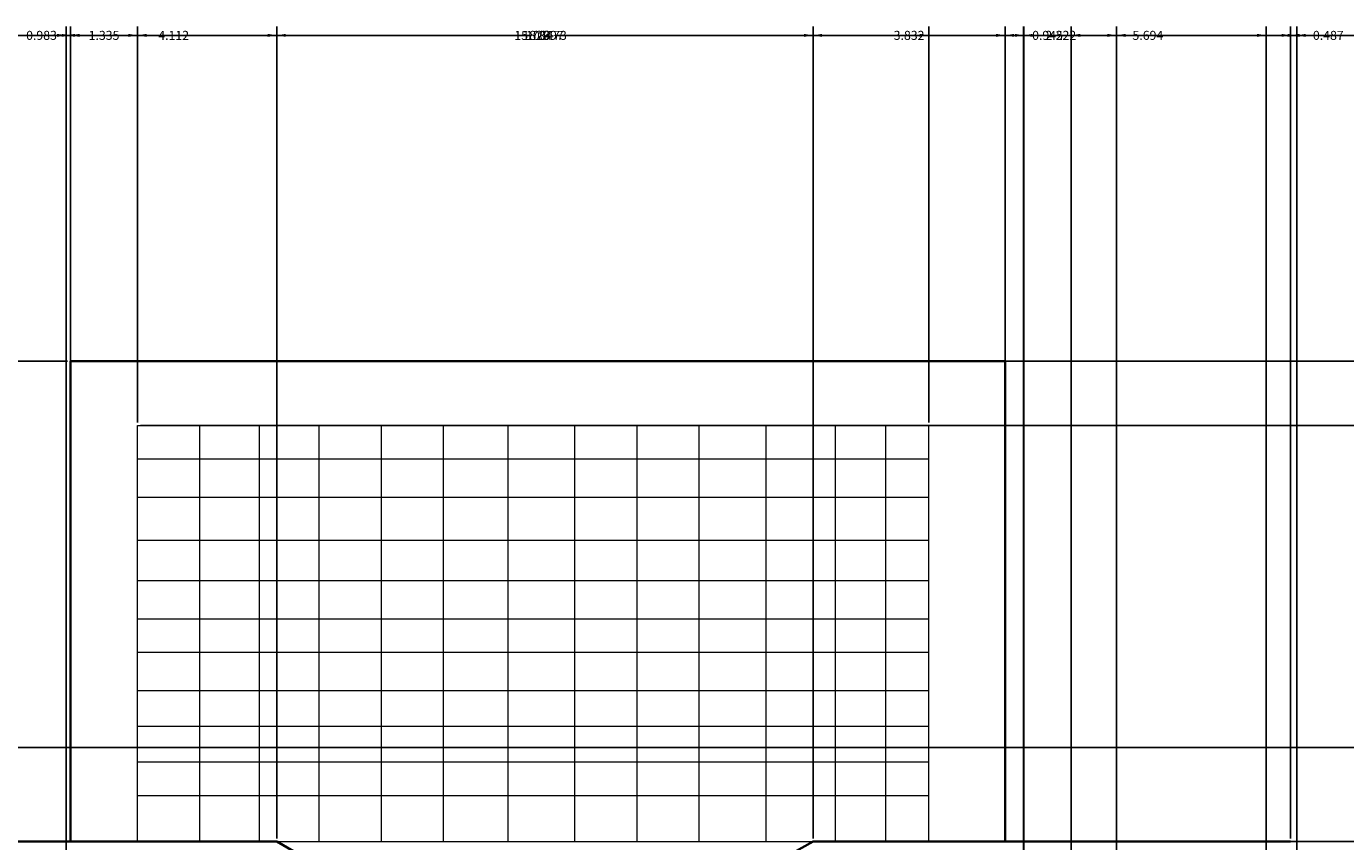
# Model space of a CAD drawing. Units: inches. Extents: x -10 to 130, y -32 to 34.
# Tile 17 of 22: x 49 to 75, y 18 to 34. Entities that reach past the tile are written whole.
import ezdxf

# ---------------------------------------------------------------- set-up
doc = ezdxf.new("R2010")
doc.units = ezdxf.units.IN
doc.header["$MEASUREMENT"] = 0
for name, color, linetype, lineweight in [('A-ANNO-DIMS', 2, 'Continuous', 18), ('A-ELEV', 7, 'Continuous', 35), ('A-GLAZ', 4, 'Continuous', 18)]:
    doc.layers.add(name, color=color, linetype=linetype, lineweight=lineweight)
doc.styles.get("Standard").update_dxf_attribs({"font": 'arial.ttf'})
doc.dimstyles.get("Standard").update_dxf_attribs({"dimtxt": 0.18, "dimasz": 0.18, "dimexe": 0.18, "dimexo": 0.0625, "dimgap": 0.09, "dimtad": 0, "dimtih": 1, "dimtoh": 1, "dimdec": 4, "dimzin": 0, "dimdsep": 46, "dimtxsty": 'Standard', "dimcen": 0.09, "dimadec": 0, "dimazin": 0, "dimtfac": 1, "dimtdec": 4, "dimtofl": 0, "dimtmove": 0, "dimatfit": 3, "dimfxl": 1, "dimtolj": 1, "dimtzin": 0, "dimarcsym": 0})

# ---------------------------------------------------------------- blocks, each defined once
blk = doc.blocks.new('*D2')
at = {"layer": 'A-ANNO-DIMS', "color": 0, "lineweight": -2, "transparency": 16777216}
for p, q in [((68.738, 27.199), (129.508, 27.199)), ((129.328, 27.019), (129.328, 3.074)), ((129.328, -21.234), (129.328, 2.71)), ((107.996, -21.414), (129.508, -21.414))]:
    blk.add_line(p, q, dxfattribs=at)
at = {"layer": 'A-ANNO-DIMS', "color": 0, "transparency": 16777216}
for points in [[(129.298, 27.019), (129.358, 27.019), (129.328, 27.199)], [(129.298, -21.234), (129.358, -21.234), (129.328, -21.414)]]:
    blk.add_solid(points, dxfattribs=at)
at = {"layer": 'Defpoints', "color": 0, "transparency": 16777216}
for p in [(68.676, 27.199), (129.328, 27.199), (107.933, -21.414)]:
    blk.add_point(p, dxfattribs=at)
at = {"layer": 'A-ANNO-DIMS', "color": 0, "transparency": 16777216, "insert": (129.328, 2.892), "char_height": 0.18, "attachment_point": 5}
blk.add_mtext('\\A1;48.61', dxfattribs=at)
blk = doc.blocks.new('*D7')
at = {"layer": 'A-ANNO-DIMS', "color": 0, "lineweight": -2, "transparency": 16777216}
for p, q in [((42.614, 6.07), (42.614, 33.879)), ((42.794, 33.699), (45.888, 33.699)), ((49.766, 33.699), (46.672, 33.699)), ((49.946, 6.07), (49.946, 33.879))]:
    blk.add_line(p, q, dxfattribs=at)
at = {"layer": 'A-ANNO-DIMS', "color": 0, "transparency": 16777216}
for points in [[(42.794, 33.729), (42.794, 33.669), (42.614, 33.699)], [(49.766, 33.729), (49.766, 33.669), (49.946, 33.699)]]:
    blk.add_solid(points, dxfattribs=at)
at = {"layer": 'Defpoints', "color": 0, "transparency": 16777216}
for p in [(49.946, 33.699), (42.614, 6.007), (49.946, 6.007)]:
    blk.add_point(p, dxfattribs=at)
at = {"layer": 'A-ANNO-DIMS', "color": 0, "transparency": 16777216, "insert": (46.28, 33.699), "char_height": 0.18, "attachment_point": 5}
blk.add_mtext('\\A1;7.332', dxfattribs=at)
blk = doc.blocks.new('*D8')
at = {"layer": 'A-ANNO-DIMS', "color": 0, "lineweight": -2, "transparency": 16777216}
for p, q in [((68.676, 17.67), (68.676, 33.879)), ((68.856, 33.699), (69.393, 33.699)), ((70.718, 33.699), (70.181, 33.699)), ((70.898, 6.07), (70.898, 33.879))]:
    blk.add_line(p, q, dxfattribs=at)
at = {"layer": 'A-ANNO-DIMS', "color": 0, "transparency": 16777216}
for points in [[(68.856, 33.729), (68.856, 33.669), (68.676, 33.699)], [(70.718, 33.729), (70.718, 33.669), (70.898, 33.699)]]:
    blk.add_solid(points, dxfattribs=at)
at = {"layer": 'Defpoints', "color": 0, "transparency": 16777216}
for p in [(70.898, 33.699), (68.676, 17.607), (70.898, 6.007)]:
    blk.add_point(p, dxfattribs=at)
at = {"layer": 'A-ANNO-DIMS', "color": 0, "transparency": 16777216, "insert": (69.787, 33.699), "char_height": 0.18, "attachment_point": 5}
blk.add_mtext('\\A1;2.222', dxfattribs=at)
blk = doc.blocks.new('*D9')
at = {"layer": 'A-ANNO-DIMS', "color": 0, "lineweight": -2, "transparency": 16777216}
for p, q in [((70.898, 6.07), (70.898, 33.879)), ((71.078, 33.699), (75.697, 33.699)), ((81.225, 33.699), (76.607, 33.699)), ((81.405, 6.07), (81.405, 33.879))]:
    blk.add_line(p, q, dxfattribs=at)
at = {"layer": 'A-ANNO-DIMS', "color": 0, "transparency": 16777216}
for points in [[(71.078, 33.729), (71.078, 33.669), (70.898, 33.699)], [(81.225, 33.729), (81.225, 33.669), (81.405, 33.699)]]:
    blk.add_solid(points, dxfattribs=at)
at = {"layer": 'Defpoints', "color": 0, "transparency": 16777216}
for p in [(81.405, 33.699), (70.898, 6.007), (81.405, 6.007)]:
    blk.add_point(p, dxfattribs=at)
at = {"layer": 'A-ANNO-DIMS', "color": 0, "transparency": 16777216, "insert": (76.152, 33.699), "char_height": 0.18, "attachment_point": 5}
blk.add_mtext('\\A1;10.507', dxfattribs=at)
blk = doc.blocks.new('*D18')
at = {"layer": 'A-ANNO-DIMS', "color": 0, "lineweight": -2, "transparency": 16777216}
for p, q in [((44.622, 17.67), (44.622, 33.879)), ((44.802, 33.699), (46.935, 33.699)), ((49.855, 33.699), (47.722, 33.699)), ((50.035, 27.261), (50.035, 33.879))]:
    blk.add_line(p, q, dxfattribs=at)
at = {"layer": 'A-ANNO-DIMS', "color": 0, "transparency": 16777216}
for points in [[(44.802, 33.729), (44.802, 33.669), (44.622, 33.699)], [(49.855, 33.729), (49.855, 33.669), (50.035, 33.699)]]:
    blk.add_solid(points, dxfattribs=at)
at = {"layer": 'Defpoints', "color": 0, "transparency": 16777216}
for p in [(50.035, 33.699), (50.035, 27.199), (44.622, 17.607)]:
    blk.add_point(p, dxfattribs=at)
at = {"layer": 'A-ANNO-DIMS', "color": 0, "transparency": 16777216, "insert": (47.328, 33.699), "char_height": 0.18, "attachment_point": 5}
blk.add_mtext('\\A1;5.413', dxfattribs=at)
blk = doc.blocks.new('*D19')
at = {"layer": 'A-ANNO-DIMS', "color": 0, "lineweight": -2, "transparency": 16777216}
for p, q in [((50.035, 27.261), (50.035, 33.879)), ((50.215, 33.699), (58.97, 33.699)), ((68.496, 33.699), (59.74, 33.699)), ((68.676, 27.261), (68.676, 33.879))]:
    blk.add_line(p, q, dxfattribs=at)
at = {"layer": 'A-ANNO-DIMS', "color": 0, "transparency": 16777216}
for points in [[(50.215, 33.729), (50.215, 33.669), (50.035, 33.699)], [(68.496, 33.729), (68.496, 33.669), (68.676, 33.699)]]:
    blk.add_solid(points, dxfattribs=at)
at = {"layer": 'Defpoints', "color": 0, "transparency": 16777216}
for p in [(68.676, 33.699), (50.035, 27.199), (68.676, 27.199)]:
    blk.add_point(p, dxfattribs=at)
at = {"layer": 'A-ANNO-DIMS', "color": 0, "transparency": 16777216, "insert": (59.355, 33.699), "char_height": 0.18, "attachment_point": 5}
blk.add_mtext('\\A1;18.64', dxfattribs=at)
blk = doc.blocks.new('*D20')
at = {"layer": 'A-ANNO-DIMS', "color": 0, "lineweight": -2, "transparency": 16777216}
for p, q in [((68.676, 27.261), (68.676, 33.879)), ((68.856, 33.699), (71.129, 33.699)), ((74.19, 33.699), (71.916, 33.699)), ((74.37, 17.67), (74.37, 33.879))]:
    blk.add_line(p, q, dxfattribs=at)
at = {"layer": 'A-ANNO-DIMS', "color": 0, "transparency": 16777216}
for points in [[(68.856, 33.729), (68.856, 33.669), (68.676, 33.699)], [(74.19, 33.729), (74.19, 33.669), (74.37, 33.699)]]:
    blk.add_solid(points, dxfattribs=at)
at = {"layer": 'Defpoints', "color": 0, "transparency": 16777216}
for p in [(74.37, 33.699), (68.676, 27.199), (74.37, 17.607)]:
    blk.add_point(p, dxfattribs=at)
at = {"layer": 'A-ANNO-DIMS', "color": 0, "transparency": 16777216, "insert": (71.523, 33.699), "char_height": 0.18, "attachment_point": 5}
blk.add_mtext('\\A1;5.694', dxfattribs=at)
blk = doc.blocks.new('*D21')
at = {"layer": 'A-ANNO-DIMS', "color": 0, "lineweight": -2, "transparency": 16777216}
for p, q in [((74.37, 17.67), (74.37, 33.879)), ((74.55, 33.699), (76.605, 33.699)), ((79.447, 33.699), (77.392, 33.699)), ((79.627, 19.52), (79.627, 33.879))]:
    blk.add_line(p, q, dxfattribs=at)
at = {"layer": 'A-ANNO-DIMS', "color": 0, "transparency": 16777216}
for points in [[(74.55, 33.729), (74.55, 33.669), (74.37, 33.699)], [(79.447, 33.729), (79.447, 33.669), (79.627, 33.699)]]:
    blk.add_solid(points, dxfattribs=at)
at = {"layer": 'Defpoints', "color": 0, "transparency": 16777216}
for p in [(79.627, 33.699), (79.627, 19.458), (74.37, 17.607)]:
    blk.add_point(p, dxfattribs=at)
at = {"layer": 'A-ANNO-DIMS', "color": 0, "transparency": 16777216, "insert": (76.998, 33.699), "char_height": 0.18, "attachment_point": 5}
blk.add_mtext('\\A1;5.257', dxfattribs=at)
blk = doc.blocks.new('*D28')
at = {"layer": 'A-ANNO-DIMS', "color": 0, "lineweight": -2, "transparency": 16777216}
for p, q in [((21.715, 14.903), (21.715, 33.879)), ((21.895, 33.699), (35.436, 33.699)), ((49.766, 33.699), (36.226, 33.699)), ((49.946, 14.903), (49.946, 33.879))]:
    blk.add_line(p, q, dxfattribs=at)
at = {"layer": 'A-ANNO-DIMS', "color": 0, "transparency": 16777216}
for points in [[(21.895, 33.729), (21.895, 33.669), (21.715, 33.699)], [(49.766, 33.729), (49.766, 33.669), (49.946, 33.699)]]:
    blk.add_solid(points, dxfattribs=at)
at = {"layer": 'Defpoints', "color": 0, "transparency": 16777216}
for p in [(49.946, 33.699), (21.715, 14.841), (49.946, 14.841)]:
    blk.add_point(p, dxfattribs=at)
at = {"layer": 'A-ANNO-DIMS', "color": 0, "transparency": 16777216, "insert": (35.831, 33.699), "char_height": 0.18, "attachment_point": 5}
blk.add_mtext('\\A1;28.23', dxfattribs=at)
blk = doc.blocks.new('*D29')
at = {"layer": 'A-ANNO-DIMS', "color": 0, "lineweight": -2, "transparency": 16777216}
for p, q in [((69.045, 14.903), (69.045, 33.879)), ((69.225, 33.699), (82.743, 33.699)), ((97.053, 33.699), (83.534, 33.699)), ((97.233, 14.903), (97.233, 33.879))]:
    blk.add_line(p, q, dxfattribs=at)
at = {"layer": 'A-ANNO-DIMS', "color": 0, "transparency": 16777216}
for points in [[(69.225, 33.729), (69.225, 33.669), (69.045, 33.699)], [(97.053, 33.729), (97.053, 33.669), (97.233, 33.699)]]:
    blk.add_solid(points, dxfattribs=at)
at = {"layer": 'Defpoints', "color": 0, "transparency": 16777216}
for p in [(97.233, 33.699), (69.045, 14.841), (97.233, 14.841)]:
    blk.add_point(p, dxfattribs=at)
at = {"layer": 'A-ANNO-DIMS', "color": 0, "transparency": 16777216, "insert": (83.139, 33.699), "char_height": 0.18, "attachment_point": 5}
blk.add_mtext('\\A1;28.19', dxfattribs=at)
blk = doc.blocks.new('*D39')
at = {"layer": 'A-ANNO-DIMS', "color": 0, "lineweight": -2, "transparency": 16777216}
for p, q in [((49.972, 27.199), (-9.564, 27.199)), ((-9.384, 27.019), (-9.384, 25.982)), ((-9.384, 24.582), (-9.384, 25.618)), ((28.037, 24.402), (-9.564, 24.402))]:
    blk.add_line(p, q, dxfattribs=at)
at = {"layer": 'A-ANNO-DIMS', "color": 0, "transparency": 16777216}
for points in [[(-9.414, 27.019), (-9.354, 27.019), (-9.384, 27.199)], [(-9.414, 24.582), (-9.354, 24.582), (-9.384, 24.402)]]:
    blk.add_solid(points, dxfattribs=at)
at = {"layer": 'Defpoints', "color": 0, "transparency": 16777216}
for p in [(-9.384, 27.199), (50.035, 27.199), (28.1, 24.402)]:
    blk.add_point(p, dxfattribs=at)
at = {"layer": 'A-ANNO-DIMS', "color": 0, "transparency": 16777216, "insert": (-9.384, 25.8), "char_height": 0.18, "attachment_point": 5}
blk.add_mtext('\\A1;2.797', dxfattribs=at)
blk = doc.blocks.new('*D48')
at = {"layer": 'A-ANNO-DIMS', "color": 0, "lineweight": -2, "transparency": 16777216}
for p, q in [((44.76, -13.293), (44.76, 33.879)), ((44.94, 33.699), (59.231, 33.699)), ((74.312, 33.699), (60.021, 33.699)), ((74.492, -13.293), (74.492, 33.879))]:
    blk.add_line(p, q, dxfattribs=at)
at = {"layer": 'A-ANNO-DIMS', "color": 0, "transparency": 16777216}
for points in [[(44.94, 33.729), (44.94, 33.669), (44.76, 33.699)], [(74.312, 33.729), (74.312, 33.669), (74.492, 33.699)]]:
    blk.add_solid(points, dxfattribs=at)
at = {"layer": 'Defpoints', "color": 0, "transparency": 16777216}
for p in [(74.492, 33.699), (44.76, -13.356), (74.492, -13.356)]:
    blk.add_point(p, dxfattribs=at)
at = {"layer": 'A-ANNO-DIMS', "color": 0, "transparency": 16777216, "insert": (59.626, 33.699), "char_height": 0.18, "attachment_point": 5}
blk.add_mtext('\\A1;29.73', dxfattribs=at)
blk = doc.blocks.new('*D60')
at = {"layer": 'A-ANNO-DIMS', "color": 0, "lineweight": -2, "transparency": 16777216}
for p, q in [((74.492, -13.293), (74.492, 33.879)), ((74.672, 33.699), (78.041, 33.699)), ((82.197, 33.699), (78.828, 33.699)), ((82.377, -15.202), (82.377, 33.879))]:
    blk.add_line(p, q, dxfattribs=at)
at = {"layer": 'A-ANNO-DIMS', "color": 0, "transparency": 16777216}
for points in [[(74.672, 33.729), (74.672, 33.669), (74.492, 33.699)], [(82.197, 33.729), (82.197, 33.669), (82.377, 33.699)]]:
    blk.add_solid(points, dxfattribs=at)
at = {"layer": 'Defpoints', "color": 0, "transparency": 16777216}
for p in [(82.377, 33.699), (74.492, -13.356), (82.377, -15.264)]:
    blk.add_point(p, dxfattribs=at)
at = {"layer": 'A-ANNO-DIMS', "color": 0, "transparency": 16777216, "insert": (78.435, 33.699), "char_height": 0.18, "attachment_point": 5}
blk.add_mtext('\\A1;7.885', dxfattribs=at)
blk = doc.blocks.new('*D70')
at = {"layer": 'A-ANNO-DIMS', "color": 0, "lineweight": -2, "transparency": 16777216}
for p, q in [((50.035, 17.67), (50.035, 33.879)), ((50.215, 33.699), (51.695, 33.699)), ((53.967, 33.699), (52.487, 33.699)), ((54.147, 17.67), (54.147, 33.879))]:
    blk.add_line(p, q, dxfattribs=at)
at = {"layer": 'A-ANNO-DIMS', "color": 0, "transparency": 16777216}
for points in [[(50.215, 33.729), (50.215, 33.669), (50.035, 33.699)], [(53.967, 33.729), (53.967, 33.669), (54.147, 33.699)]]:
    blk.add_solid(points, dxfattribs=at)
at = {"layer": 'Defpoints', "color": 0, "transparency": 16777216}
for p in [(54.147, 33.699), (50.035, 17.607), (54.147, 17.607)]:
    blk.add_point(p, dxfattribs=at)
at = {"layer": 'A-ANNO-DIMS', "color": 0, "transparency": 16777216, "insert": (52.091, 33.699), "char_height": 0.18, "attachment_point": 5}
blk.add_mtext('\\A1;4.112', dxfattribs=at)
blk = doc.blocks.new('*D71')
at = {"layer": 'A-ANNO-DIMS', "color": 0, "lineweight": -2, "transparency": 16777216}
for p, q in [((54.147, 17.67), (54.147, 33.879)), ((54.327, 33.699), (59.041, 33.699)), ((64.664, 33.699), (59.951, 33.699)), ((64.844, 17.67), (64.844, 33.879))]:
    blk.add_line(p, q, dxfattribs=at)
at = {"layer": 'A-ANNO-DIMS', "color": 0, "transparency": 16777216}
for points in [[(54.327, 33.729), (54.327, 33.669), (54.147, 33.699)], [(64.664, 33.729), (64.664, 33.669), (64.844, 33.699)]]:
    blk.add_solid(points, dxfattribs=at)
at = {"layer": 'Defpoints', "color": 0, "transparency": 16777216}
for p in [(64.844, 33.699), (54.147, 17.607), (64.844, 17.607)]:
    blk.add_point(p, dxfattribs=at)
at = {"layer": 'A-ANNO-DIMS', "color": 0, "transparency": 16777216, "insert": (59.496, 33.699), "char_height": 0.18, "attachment_point": 5}
blk.add_mtext('\\A1;10.697', dxfattribs=at)
blk = doc.blocks.new('*D74')
at = {"layer": 'A-ANNO-DIMS', "color": 0, "lineweight": -2, "transparency": 16777216}
for p, q in [((54.085, 17.607), (-9.564, 17.607)), ((-9.384, 17.427), (-9.384, 17.281)), ((-9.384, 16.771), (-9.384, 16.917)), ((55.856, 16.591), (-9.564, 16.591))]:
    blk.add_line(p, q, dxfattribs=at)
at = {"layer": 'A-ANNO-DIMS', "color": 0, "transparency": 16777216}
for points in [[(-9.414, 17.427), (-9.354, 17.427), (-9.384, 17.607)], [(-9.414, 16.771), (-9.354, 16.771), (-9.384, 16.591)]]:
    blk.add_solid(points, dxfattribs=at)
at = {"layer": 'Defpoints', "color": 0, "transparency": 16777216}
for p in [(54.147, 17.607), (-9.384, 16.591), (55.918, 16.591)]:
    blk.add_point(p, dxfattribs=at)
at = {"layer": 'A-ANNO-DIMS', "color": 0, "transparency": 16777216, "insert": (-9.384, 17.099), "char_height": 0.18, "attachment_point": 5}
blk.add_mtext('\\A1;1.02', dxfattribs=at)
blk = doc.blocks.new('*D82')
at = {"layer": 'A-ANNO-DIMS', "color": 0, "lineweight": -2, "transparency": 16777216}
for p, q in [((19.651, 19.485), (129.508, 19.485)), ((129.328, 19.305), (129.328, 18.728)), ((129.328, 17.787), (129.328, 18.364)), ((68.738, 17.607), (129.508, 17.607))]:
    blk.add_line(p, q, dxfattribs=at)
at = {"layer": 'A-ANNO-DIMS', "color": 0, "transparency": 16777216}
for points in [[(129.298, 19.305), (129.358, 19.305), (129.328, 19.485)], [(129.298, 17.787), (129.358, 17.787), (129.328, 17.607)]]:
    blk.add_solid(points, dxfattribs=at)
at = {"layer": 'Defpoints', "color": 0, "transparency": 16777216}
for p in [(19.588, 19.485), (68.676, 17.607), (129.328, 17.607)]:
    blk.add_point(p, dxfattribs=at)
at = {"layer": 'A-ANNO-DIMS', "color": 0, "transparency": 16777216, "insert": (129.328, 18.546), "char_height": 0.18, "attachment_point": 5}
blk.add_mtext('\\A1;1.877', dxfattribs=at)
blk = doc.blocks.new('*D83')
at = {"layer": 'A-ANNO-DIMS', "color": 0, "lineweight": -2, "transparency": 16777216}
for p, q in [((50.035, 27.261), (50.035, 33.879)), ((50.215, 33.699), (50.316, 33.699)), ((51.19, 33.699), (51.088, 33.699)), ((51.37, 25.975), (51.37, 33.879))]:
    blk.add_line(p, q, dxfattribs=at)
at = {"layer": 'A-ANNO-DIMS', "color": 0, "transparency": 16777216}
for points in [[(50.215, 33.729), (50.215, 33.669), (50.035, 33.699)], [(51.19, 33.729), (51.19, 33.669), (51.37, 33.699)]]:
    blk.add_solid(points, dxfattribs=at)
at = {"layer": 'Defpoints', "color": 0, "transparency": 16777216}
for p in [(51.37, 33.699), (50.035, 27.199), (51.37, 25.913)]:
    blk.add_point(p, dxfattribs=at)
at = {"layer": 'A-ANNO-DIMS', "color": 0, "transparency": 16777216, "insert": (50.702, 33.699), "char_height": 0.18, "attachment_point": 5}
blk.add_mtext('\\A1;1.335', dxfattribs=at)
blk = doc.blocks.new('*D84')
at = {"layer": 'A-ANNO-DIMS', "color": 0, "lineweight": -2, "transparency": 16777216}
for p, q in [((51.37, 25.975), (51.37, 33.879)), ((51.55, 33.699), (58.807, 33.699)), ((66.974, 33.699), (59.717, 33.699)), ((67.154, 25.975), (67.154, 33.879))]:
    blk.add_line(p, q, dxfattribs=at)
at = {"layer": 'A-ANNO-DIMS', "color": 0, "transparency": 16777216}
for points in [[(51.55, 33.729), (51.55, 33.669), (51.37, 33.699)], [(66.974, 33.729), (66.974, 33.669), (67.154, 33.699)]]:
    blk.add_solid(points, dxfattribs=at)
at = {"layer": 'Defpoints', "color": 0, "transparency": 16777216}
for p in [(67.154, 33.699), (51.37, 25.913), (67.154, 25.913)]:
    blk.add_point(p, dxfattribs=at)
at = {"layer": 'A-ANNO-DIMS', "color": 0, "transparency": 16777216, "insert": (59.262, 33.699), "char_height": 0.18, "attachment_point": 5}
blk.add_mtext('\\A1;15.784', dxfattribs=at)
blk = doc.blocks.new('*D85')
at = {"layer": 'A-ANNO-DIMS', "color": 0, "lineweight": -2, "transparency": 16777216}
for p, q in [((50.097, 27.199), (129.508, 27.199)), ((129.328, 27.019), (129.328, 26.738)), ((129.328, 26.093), (129.328, 26.374)), ((51.432, 25.913), (129.508, 25.913))]:
    blk.add_line(p, q, dxfattribs=at)
at = {"layer": 'A-ANNO-DIMS', "color": 0, "transparency": 16777216}
for points in [[(129.298, 27.019), (129.358, 27.019), (129.328, 27.199)], [(129.298, 26.093), (129.358, 26.093), (129.328, 25.913)]]:
    blk.add_solid(points, dxfattribs=at)
at = {"layer": 'Defpoints', "color": 0, "transparency": 16777216}
for p in [(50.035, 27.199), (129.328, 27.199), (51.37, 25.913)]:
    blk.add_point(p, dxfattribs=at)
at = {"layer": 'A-ANNO-DIMS', "color": 0, "transparency": 16777216, "insert": (129.328, 26.556), "char_height": 0.18, "attachment_point": 5}
blk.add_mtext('\\A1;1.286', dxfattribs=at)
blk = doc.blocks.new('*D86')
at = {"layer": 'A-ANNO-DIMS', "color": 0, "lineweight": -2, "transparency": 16777216}
for p, q in [((64.844, 17.67), (64.844, 33.879)), ((65.024, 33.699), (66.367, 33.699)), ((68.496, 33.699), (67.153, 33.699)), ((68.676, 17.67), (68.676, 33.879))]:
    blk.add_line(p, q, dxfattribs=at)
at = {"layer": 'A-ANNO-DIMS', "color": 0, "transparency": 16777216}
for points in [[(65.024, 33.729), (65.024, 33.669), (64.844, 33.699)], [(68.496, 33.729), (68.496, 33.669), (68.676, 33.699)]]:
    blk.add_solid(points, dxfattribs=at)
at = {"layer": 'Defpoints', "color": 0, "transparency": 16777216}
for p in [(68.676, 33.699), (64.844, 17.607), (68.676, 17.607)]:
    blk.add_point(p, dxfattribs=at)
at = {"layer": 'A-ANNO-DIMS', "color": 0, "transparency": 16777216, "insert": (66.76, 33.699), "char_height": 0.18, "attachment_point": 5}
blk.add_mtext('\\A1;3.832', dxfattribs=at)
blk = doc.blocks.new('*D107')
at = {"layer": 'A-ANNO-DIMS', "color": 0, "lineweight": -2, "transparency": 16777216}
for p, q in [((48.783, 33.699), (48.603, 33.699)), ((48.963, 14.318), (48.963, 33.879)), ((49.946, 14.903), (49.946, 33.879)), ((50.126, 33.699), (50.306, 33.699))]:
    blk.add_line(p, q, dxfattribs=at)
at = {"layer": 'A-ANNO-DIMS', "color": 0, "transparency": 16777216}
for points in [[(48.783, 33.729), (48.783, 33.669), (48.963, 33.699)], [(50.126, 33.729), (50.126, 33.669), (49.946, 33.699)]]:
    blk.add_solid(points, dxfattribs=at)
at = {"layer": 'Defpoints', "color": 0, "transparency": 16777216}
for p in [(49.946, 33.699), (49.946, 14.841), (48.963, 14.256)]:
    blk.add_point(p, dxfattribs=at)
at = {"layer": 'A-ANNO-DIMS', "color": 0, "transparency": 16777216, "insert": (49.455, 33.699), "char_height": 0.18, "attachment_point": 5}
blk.add_mtext('\\A1;0.983', dxfattribs=at)
blk = doc.blocks.new('*D136')
at = {"layer": 'A-ANNO-DIMS', "color": 0, "lineweight": -2, "transparency": 16777216}
for p, q in [((68.87, 33.699), (68.69, 33.699)), ((69.05, 14.903), (69.05, 33.879)), ((69.995, 14.206), (69.995, 33.879)), ((70.175, 33.699), (70.355, 33.699))]:
    blk.add_line(p, q, dxfattribs=at)
at = {"layer": 'A-ANNO-DIMS', "color": 0, "transparency": 16777216}
for points in [[(68.87, 33.729), (68.87, 33.669), (69.05, 33.699)], [(70.175, 33.729), (70.175, 33.669), (69.995, 33.699)]]:
    blk.add_solid(points, dxfattribs=at)
at = {"layer": 'Defpoints', "color": 0, "transparency": 16777216}
for p in [(69.995, 33.699), (69.05, 14.841), (69.995, 14.144)]:
    blk.add_point(p, dxfattribs=at)
at = {"layer": 'A-ANNO-DIMS', "color": 0, "transparency": 16777216, "insert": (69.522, 33.699), "char_height": 0.18, "attachment_point": 5}
blk.add_mtext('\\A1;0.945', dxfattribs=at)
blk = doc.blocks.new('*D137')
at = {"layer": 'A-ANNO-DIMS', "color": 0, "lineweight": -2, "transparency": 16777216}
for p, q in [((69.995, 14.206), (69.995, 33.879)), ((70.175, 33.699), (82.678, 33.699)), ((96.113, 33.699), (83.609, 33.699)), ((96.293, 14.206), (96.293, 33.879))]:
    blk.add_line(p, q, dxfattribs=at)
at = {"layer": 'A-ANNO-DIMS', "color": 0, "transparency": 16777216}
for points in [[(70.175, 33.729), (70.175, 33.669), (69.995, 33.699)], [(96.113, 33.729), (96.113, 33.669), (96.293, 33.699)]]:
    blk.add_solid(points, dxfattribs=at)
at = {"layer": 'Defpoints', "color": 0, "transparency": 16777216}
for p in [(96.293, 33.699), (69.995, 14.144), (96.293, 14.144)]:
    blk.add_point(p, dxfattribs=at)
at = {"layer": 'A-ANNO-DIMS', "color": 0, "transparency": 16777216, "insert": (83.144, 33.699), "char_height": 0.18, "attachment_point": 5}
blk.add_mtext('\\A1;26.298', dxfattribs=at)
blk = doc.blocks.new('*D149')
at = {"layer": 'A-ANNO-DIMS', "color": 0, "lineweight": -2, "transparency": 16777216}
for p, q in [((73.702, 33.699), (73.522, 33.699)), ((73.882, 17.205), (73.882, 33.879)), ((74.37, 17.67), (74.37, 33.879)), ((74.55, 33.699), (74.73, 33.699))]:
    blk.add_line(p, q, dxfattribs=at)
at = {"layer": 'A-ANNO-DIMS', "color": 0, "transparency": 16777216}
for points in [[(73.702, 33.729), (73.702, 33.669), (73.882, 33.699)], [(74.55, 33.729), (74.55, 33.669), (74.37, 33.699)]]:
    blk.add_solid(points, dxfattribs=at)
at = {"layer": 'Defpoints', "color": 0, "transparency": 16777216}
for p in [(74.37, 33.699), (74.37, 17.607), (73.882, 17.143)]:
    blk.add_point(p, dxfattribs=at)
at = {"layer": 'A-ANNO-DIMS', "color": 0, "transparency": 16777216, "insert": (75.123, 33.699), "char_height": 0.18, "attachment_point": 5}
blk.add_mtext('\\A1;0.487', dxfattribs=at)
blk = doc.blocks.new('*D150')
at = {"layer": 'A-ANNO-DIMS', "color": 0, "lineweight": -2, "transparency": 16777216}
for p, q in [((129.327673, 17.787359), (129.327673, 17.967359)), ((74.432221, 17.607359), (129.507673, 17.607359)), ((73.944831, 17.142679), (129.507673, 17.142679)), ((129.327673, 16.962679), (129.327673, 16.782679))]:
    blk.add_line(p, q, dxfattribs=at)
at = {"layer": 'A-ANNO-DIMS', "color": 0, "transparency": 16777216}
for points in [[(129.297673, 17.787359), (129.357673, 17.787359), (129.327673, 17.607359)], [(129.297673, 16.962679), (129.357673, 16.962679), (129.327673, 17.142679)]]:
    blk.add_solid(points, dxfattribs=at)
at = {"layer": 'Defpoints', "color": 0, "transparency": 16777216}
for p in [(74.369721, 17.607359), (129.327673, 17.607359), (73.882331, 17.142679)]:
    blk.add_point(p, dxfattribs=at)
at = {"layer": 'A-ANNO-DIMS', "color": 0, "transparency": 16777216, "insert": (129.327673, 17.375019), "char_height": 0.18, "attachment_point": 5}
blk.add_mtext('\\A1;0.465', dxfattribs=at)

msp = doc.modelspace()

# ---------------------------------------------------------------- linework, layer by layer
at = {"layer": 'A-ELEV'}
for p, q in [((50.0347, 17.6074), (50.0347, 27.1987)), ((50.0347, 27.1987), (68.6759, 27.1987)), ((68.6759, 27.1987), (68.6759, 17.6074)), ((44.6217, 17.6074), (54.1471, 17.6074)), ((56.395, 16.3174), (54.1471, 17.6074)), ((62.5256, 16.3174), (64.8443, 17.6074)), ((74.3697, 17.6074), (64.8443, 17.6074))]:
    msp.add_line(p, q, dxfattribs=at)
at = {"layer": 'A-GLAZ'}
for p, q in [((51.3699, 17.6074), (51.3699, 25.9127)), ((51.3699, 25.9127), (67.154, 25.9127)), ((52.6098, 17.6074), (52.6098, 25.9127)), ((53.8019, 17.6074), (53.8019, 25.9127)), ((54.9941, 17.6074), (54.9941, 25.9127)), ((56.2339, 17.6074), (56.2339, 25.9127)), ((57.4737, 17.6074), (57.4737, 25.9127)), ((58.7612, 17.6074), (58.7612, 25.9127)), ((60.0964, 17.6074), (60.0964, 25.9127)), ((61.3363, 17.6074), (61.3363, 25.9127)), ((62.5761, 17.6074), (62.5761, 25.9127)), ((63.9113, 17.6074), (63.9113, 25.9127)), ((65.2942, 17.6074), (65.2942, 25.9127)), ((66.2956, 17.6074), (66.2956, 25.9127)), ((67.154, 17.6074), (67.154, 25.9127)), ((51.3699, 25.2459), (67.154, 25.2459)), ((51.3699, 24.4838), (67.154, 24.4838)), ((51.3699, 23.6265), (67.154, 23.6265)), ((51.3699, 22.8168), (67.154, 22.8168)), ((51.3699, 22.0547), (67.154, 22.0547)), ((51.3699, 21.3879), (67.154, 21.3879)), ((51.3699, 20.6259), (67.154, 20.6259)), ((51.3699, 19.9114), (67.154, 19.9114)), ((51.3699, 19.197), (67.154, 19.197)), ((51.3699, 18.5302), (67.154, 18.5302)), ((54.1471, 17.6074), (64.8443, 17.6074))]:
    msp.add_line(p, q, dxfattribs=at)

# ---------------------------------------------------------------- dimensions: what is measured, and where the dimension line sits
at = {"layer": 'A-ANNO-DIMS'}
for base, p1, p2, override, picture, middle in [((49.9462, 33.6987), (21.7155, 14.8409), (49.9462, 14.8409), {"dimdec": 2, "dimlfac": 1, "dimrnd": 0, "dimzin": 0, "dimdsep": 46, "dimlunit": 2}, '*D28', (35.8308, 33.6987)), ((49.9462, 33.6987), (42.614, 6.0074), (49.9462, 6.0074), {"dimdec": 3, "dimlfac": 1, "dimrnd": 0, "dimzin": 0, "dimdsep": 46, "dimlunit": 2}, '*D7', (46.2801, 33.6987)), ((50.0347, 33.6987), (44.6217, 17.6074), (50.0347, 27.1987), {"dimdec": 3, "dimlfac": 1, "dimrnd": 0, "dimzin": 0, "dimdsep": 46, "dimlunit": 2}, '*D18', (47.3282, 33.6987)), ((74.492, 33.6987), (44.76, -13.3558), (74.492, -13.3558), {"dimdec": 2, "dimlfac": 1, "dimrnd": 0, "dimzin": 0, "dimdsep": 46, "dimlunit": 2}, '*D48', (59.626, 33.6987)), ((49.9462, 33.6987), (48.963, 14.2556), (49.9462, 14.8409), {"dimdec": 3, "dimlfac": 1, "dimrnd": 0, "dimzin": 0, "dimdsep": 46, "dimlunit": 2}, '*D107', (49.4546, 33.6987)), ((68.6759, 33.6987), (50.0347, 27.1987), (68.6759, 27.1987), {"dimdec": 2, "dimlfac": 1, "dimrnd": 0, "dimzin": 0, "dimdsep": 46, "dimlunit": 2}, '*D19', (59.3553, 33.6987)), ((54.1471, 33.6987), (50.0347, 17.6074), (54.1471, 17.6074), {"dimdec": 3, "dimlfac": 1, "dimrnd": 0, "dimzin": 0, "dimdsep": 46, "dimlunit": 2}, '*D70', (52.0909, 33.6987)), ((51.3699, 33.6987), (50.0347, 27.1987), (51.3699, 25.9127), {"dimdec": 3, "dimlfac": 1, "dimrnd": 0, "dimzin": 0, "dimdsep": 46, "dimlunit": 2}, '*D83', (50.7023, 33.6987)), ((67.154, 33.6987), (51.3699, 25.9127), (67.154, 25.9127), {"dimdec": 3, "dimlfac": 1, "dimrnd": 0, "dimzin": 0, "dimdsep": 46, "dimlunit": 2}, '*D84', (59.2619, 33.6987)), ((64.8443, 33.6987), (54.1471, 17.6074), (64.8443, 17.6074), {"dimdec": 3, "dimlfac": 1, "dimrnd": 0, "dimzin": 0, "dimdsep": 46, "dimlunit": 2}, '*D71', (59.4957, 33.6987)), ((68.6759, 33.6987), (64.8443, 17.6074), (68.6759, 17.6074), {"dimdec": 3, "dimlfac": 1, "dimrnd": 0, "dimzin": 0, "dimdsep": 46, "dimlunit": 2}, '*D86', (66.7601, 33.6987)), ((70.898, 33.6987), (68.6759, 17.6074), (70.898, 6.0074), {"dimdec": 3, "dimlfac": 1, "dimrnd": 0, "dimzin": 0, "dimdsep": 46, "dimlunit": 2}, '*D8', (69.7869, 33.6987)), ((74.3697, 33.6987), (68.6759, 27.1987), (74.3697, 17.6074), {"dimdec": 3, "dimlfac": 1, "dimrnd": 0, "dimzin": 0, "dimdsep": 46, "dimlunit": 2}, '*D20', (71.5228, 33.6987)), ((69.9946, 33.6987), (69.0498, 14.8409), (69.9946, 14.144), {"dimdec": 3, "dimlfac": 1, "dimrnd": 0, "dimzin": 0, "dimdsep": 46, "dimlunit": 2}, '*D136', (69.5222, 33.6987)), ((97.2325, 33.6987), (69.0452, 14.8409), (97.2325, 14.8409), {"dimdec": 2, "dimlfac": 1, "dimrnd": 0, "dimzin": 0, "dimdsep": 46, "dimlunit": 2}, '*D29', (83.1389, 33.6987)), ((96.2927, 33.6987), (69.9946, 14.144), (96.2927, 14.144), {"dimdec": 3, "dimlfac": 1, "dimrnd": 0, "dimzin": 0, "dimdsep": 46, "dimlunit": 2}, '*D137', (83.1437, 33.6987)), ((81.4053, 33.6987), (70.898, 6.0074), (81.4053, 6.0074), {"dimdec": 3, "dimlfac": 1, "dimrnd": 0, "dimzin": 0, "dimdsep": 46, "dimlunit": 2}, '*D9', (76.1517, 33.6987)), ((74.3697, 33.6987), (73.8823, 17.1427), (74.3697, 17.6074), {"dimdec": 3, "dimlfac": 1, "dimrnd": 0, "dimzin": 0, "dimdsep": 46, "dimlunit": 2}, '*D149', (75.1234, 33.6987)), ((79.627, 33.6987), (74.3697, 17.6074), (79.627, 19.4575), {"dimdec": 3, "dimlfac": 1, "dimrnd": 0, "dimzin": 0, "dimdsep": 46, "dimlunit": 2}, '*D21', (76.9984, 33.6987)), ((82.377, 33.6987), (74.492, -13.3558), (82.377, -15.2645), {"dimdec": 3, "dimlfac": 1, "dimrnd": 0, "dimzin": 0, "dimdsep": 46, "dimlunit": 2}, '*D60', (78.4345, 33.6987))]:
    dim = msp.add_linear_dim(base=base, p1=p1, p2=p2, dimstyle='Standard', override=override, dxfattribs=at)
    dim.commit()
    dim.dimension.update_dxf_attribs({"geometry": picture, "text_midpoint": middle})
for base, p1, p2, override, picture, middle in [((-9.3836, 27.1987), (28.0997, 24.4019), (50.0347, 27.1987), {"dimdec": 3, "dimlfac": 1, "dimrnd": 0, "dimzin": 0, "dimdsep": 46, "dimlunit": 2}, '*D39', (-9.3836, 25.8003)), ((129.3277, 27.1987), (51.3699, 25.9127), (50.0347, 27.1987), {"dimdec": 3, "dimlfac": 1, "dimrnd": 0, "dimzin": 0, "dimdsep": 46, "dimlunit": 2}, '*D85', (129.3277, 26.5557)), ((129.3277, 27.1987), (107.9333, -21.4145), (68.6759, 27.1987), {"dimdec": 2, "dimlfac": 1, "dimrnd": 0, "dimzin": 0, "dimdsep": 46, "dimlunit": 2}, '*D2', (129.3277, 2.8921)), ((129.3277, 17.6074), (19.5881, 19.4845), (68.6759, 17.6074), {"dimdec": 3, "dimlfac": 1, "dimrnd": 0, "dimzin": 0, "dimdsep": 46, "dimlunit": 2}, '*D82', (129.3277, 18.5459)), ((129.3277, 17.6074), (73.8823, 17.1427), (74.3697, 17.6074), {"dimdec": 3, "dimlfac": 1, "dimrnd": 0, "dimzin": 0, "dimdsep": 46, "dimlunit": 2}, '*D150', (129.3277, 17.375)), ((-9.3836, 16.5911), (54.1471, 17.6074), (55.9182, 16.5911), {"dimdec": 2, "dimlfac": 1, "dimrnd": 0, "dimzin": 0, "dimdsep": 46, "dimlunit": 2}, '*D74', (-9.3836, 17.0992))]:
    dim = msp.add_linear_dim(base=base, p1=p1, p2=p2, angle=90, dimstyle='Standard', override=override, dxfattribs=at)
    dim.commit()
    dim.dimension.update_dxf_attribs({"geometry": picture, "text_midpoint": middle})

doc.saveas('drawing.dxf')
